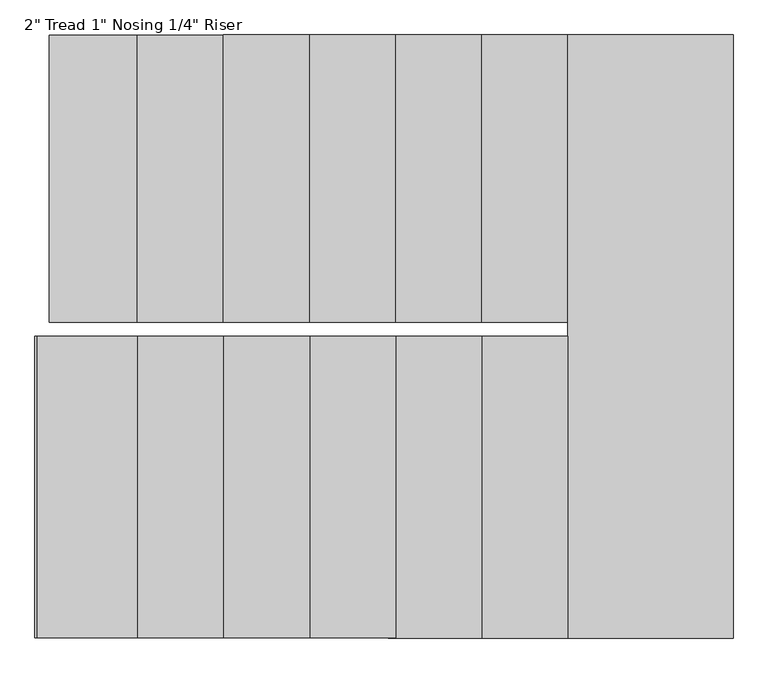
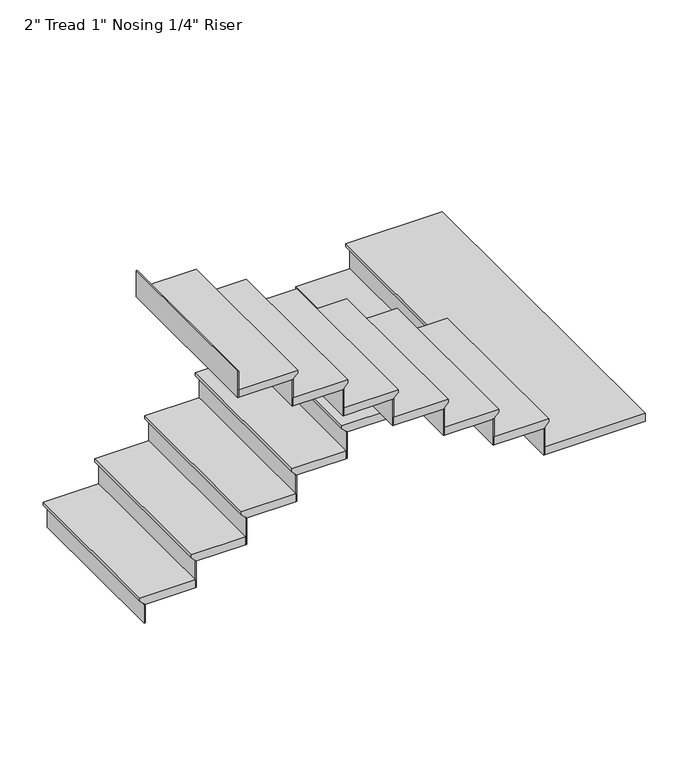
"""IFC4 building model written with IfcOpenShell, lengths in millimetres: stair flight geometry."""

from ifc_helpers import new_model, si_unit, origin, place, context, project, spatial, faceted_brep, source, transform, mapped, element, save


def stair_flight_5b4b54c9(model_context):
    return source(origin(), model_context, "Body", "Brep", [
        faceted_brep([(-1167.6638307, -167.7482799, 150.2833333), (-1167.6638307, -167.7482799, 169.3333333), (-1167.6638307, 848.2517201, 169.3333333), (-1167.6638307, 848.2517201, 150.2833333), (-1142.2638307, -167.7482799, 124.8833333), (-1142.2638307, 848.2517201, 124.8833333), (-831.1138307, -167.7482799, 169.3333333), (-831.1138307, 848.2517201, 169.3333333), (-1142.2638307, 848.2517201, 118.5333333), (-831.1138307, 848.2517201, 118.5333333), (-831.1138307, -167.7482799, 118.5333333), (-1142.2638307, -167.7482799, 118.5333333)], [[[0, 1, 2, 3]], [[4, 0, 3, 5]], [[2, 1, 6, 7]], [[8, 9, 10, 11]], [[2, 7, 9, 8, 5, 3]], [[8, 11, 4, 5]], [[6, 1, 0, 4, 11, 10]], [[7, 6, 10, 9]]]),
        faceted_brep([(-1142.2638307, -167.7482799, 118.5333333), (-1142.2638307, -167.7482799, 0.0), (-1135.9138307, -167.7482799, 0.0), (-1135.9138307, -167.7482799, 118.5333333), (-1142.2638307, 848.2517201, 118.5333333), (-1135.9138307, 848.2517201, 118.5333333), (-1135.9138307, 848.2517201, 0.0), (-1142.2638307, 848.2517201, 0.0)], [[[0, 1, 2, 3]], [[4, 5, 6, 7]], [[1, 0, 4, 7]], [[2, 1, 7, 6]], [[3, 2, 6, 5]], [[0, 3, 5, 4]]]),
        faceted_brep([(-831.1138307, -167.7482799, 287.8666667), (-831.1138307, -167.7482799, 118.5333333), (-824.7638307, -167.7482799, 118.5333333), (-824.7638307, -167.7482799, 287.8666667), (-831.1138307, 848.2517201, 287.8666667), (-824.7638307, 848.2517201, 287.8666667), (-824.7638307, 848.2517201, 118.5333333), (-831.1138307, 848.2517201, 118.5333333)], [[[0, 1, 2, 3]], [[4, 5, 6, 7]], [[1, 0, 4, 7]], [[2, 1, 7, 6]], [[3, 2, 6, 5]], [[0, 3, 5, 4]]]),
        faceted_brep([(-856.5138307, 848.2517201, 338.6666667), (-856.5138307, -167.7482799, 338.6666667), (-526.3138307, -167.7482799, 338.6666667), (-526.3138307, 848.2517201, 338.6666667), (-831.1138307, 848.2517201, 287.8666667), (-526.3138307, 848.2517201, 287.8666667), (-526.3138307, -167.7482799, 287.8666667), (-831.1138307, -167.7482799, 287.8666667), (-831.1138307, 848.2517201, 294.2166667), (-856.5138307, 848.2517201, 319.6166667), (-831.1138307, -167.7482799, 294.2166667), (-856.5138307, -167.7482799, 319.6166667)], [[[0, 1, 2, 3]], [[4, 5, 6, 7]], [[0, 3, 5, 4, 8, 9]], [[4, 7, 10, 8]], [[2, 1, 11, 10, 7, 6]], [[3, 2, 6, 5]], [[11, 1, 0, 9]], [[10, 11, 9, 8]]]),
        faceted_brep([(-526.3138307, -167.7482799, 457.2), (-526.3138307, -167.7482799, 287.8666667), (-519.9638307, -167.7482799, 287.8666667), (-519.9638307, -167.7482799, 457.2), (-526.3138307, 848.2517201, 457.2), (-519.9638307, 848.2517201, 457.2), (-519.9638307, 848.2517201, 287.8666667), (-526.3138307, 848.2517201, 287.8666667)], [[[0, 1, 2, 3]], [[4, 5, 6, 7]], [[1, 0, 4, 7]], [[2, 1, 7, 6]], [[3, 2, 6, 5]], [[0, 3, 5, 4]]]),
        faceted_brep([(-551.7138307, 848.2517201, 508.0), (-551.7138307, -167.7482799, 508.0), (-221.5138307, -167.7482799, 508.0), (-221.5138307, 848.2517201, 508.0), (-526.3138307, 848.2517201, 457.2), (-221.5138307, 848.2517201, 457.2), (-221.5138307, -167.7482799, 457.2), (-526.3138307, -167.7482799, 457.2), (-526.3138307, 848.2517201, 463.55), (-551.7138307, 848.2517201, 488.95), (-526.3138307, -167.7482799, 463.55), (-551.7138307, -167.7482799, 488.95)], [[[0, 1, 2, 3]], [[4, 5, 6, 7]], [[0, 3, 5, 4, 8, 9]], [[4, 7, 10, 8]], [[2, 1, 11, 10, 7, 6]], [[3, 2, 6, 5]], [[11, 1, 0, 9]], [[10, 11, 9, 8]]]),
        faceted_brep([(-221.5138307, -167.7482799, 626.5333333), (-221.5138307, -167.7482799, 457.2), (-215.1638307, -167.7482799, 457.2), (-215.1638307, -167.7482799, 626.5333333), (-221.5138307, 848.2517201, 626.5333333), (-215.1638307, 848.2517201, 626.5333333), (-215.1638307, 848.2517201, 457.2), (-221.5138307, 848.2517201, 457.2)], [[[0, 1, 2, 3]], [[4, 5, 6, 7]], [[1, 0, 4, 7]], [[2, 1, 7, 6]], [[3, 2, 6, 5]], [[0, 3, 5, 4]]]),
        faceted_brep([(-246.9138307, 848.2517201, 677.3333333), (-246.9138307, -167.7482799, 677.3333333), (83.2861693, -167.7482799, 677.3333333), (83.2861693, 848.2517201, 677.3333333), (-221.5138307, 848.2517201, 626.5333333), (83.2861693, 848.2517201, 626.5333333), (83.2861693, -167.7482799, 626.5333333), (-221.5138307, -167.7482799, 626.5333333), (-221.5138307, 848.2517201, 632.8833333), (-246.9138307, 848.2517201, 658.2833333), (-221.5138307, -167.7482799, 632.8833333), (-246.9138307, -167.7482799, 658.2833333)], [[[0, 1, 2, 3]], [[4, 5, 6, 7]], [[0, 3, 5, 4, 8, 9]], [[4, 7, 10, 8]], [[2, 1, 11, 10, 7, 6]], [[3, 2, 6, 5]], [[11, 1, 0, 9]], [[10, 11, 9, 8]]]),
        faceted_brep([(83.2861693, -167.7482799, 795.8666667), (83.2861693, -167.7482799, 626.5333333), (89.6361693, -167.7482799, 626.5333333), (89.6361693, -167.7482799, 795.8666667), (83.2861693, 848.2517201, 795.8666667), (89.6361693, 848.2517201, 795.8666667), (89.6361693, 848.2517201, 626.5333333), (83.2861693, 848.2517201, 626.5333333)], [[[0, 1, 2, 3]], [[4, 5, 6, 7]], [[1, 0, 4, 7]], [[2, 1, 7, 6]], [[3, 2, 6, 5]], [[0, 3, 5, 4]]]),
        faceted_brep([(57.8861693, 848.2517201, 846.6666667), (57.8861693, -167.7482799, 846.6666667), (388.0861693, -167.7482799, 846.6666667), (388.0861693, 848.2517201, 846.6666667), (83.2861693, 848.2517201, 795.8666667), (388.0861693, 848.2517201, 795.8666667), (388.0861693, -167.7482799, 795.8666667), (83.2861693, -167.7482799, 795.8666667), (83.2861693, 848.2517201, 802.2166667), (57.8861693, 848.2517201, 827.6166667), (83.2861693, -167.7482799, 802.2166667), (57.8861693, -167.7482799, 827.6166667)], [[[0, 1, 2, 3]], [[4, 5, 6, 7]], [[0, 3, 5, 4, 8, 9]], [[4, 7, 10, 8]], [[2, 1, 11, 10, 7, 6]], [[3, 2, 6, 5]], [[11, 1, 0, 9]], [[10, 11, 9, 8]]]),
        faceted_brep([(388.0861693, -167.7482799, 965.2), (388.0861693, -167.7482799, 795.8666667), (394.4361693, -167.7482799, 795.8666667), (394.4361693, -167.7482799, 965.2), (388.0861693, 848.2517201, 965.2), (394.4361693, 848.2517201, 965.2), (394.4361693, 848.2517201, 795.8666667), (388.0861693, 848.2517201, 795.8666667)], [[[0, 1, 2, 3]], [[4, 5, 6, 7]], [[1, 0, 4, 7]], [[2, 1, 7, 6]], [[3, 2, 6, 5]], [[0, 3, 5, 4]]]),
        faceted_brep([(362.6861693, 848.2517201, 1016.0), (362.6861693, -167.7482799, 1016.0), (692.8861693, -167.7482799, 1016.0), (692.8861693, 848.2517201, 1016.0), (388.0861693, 848.2517201, 965.2), (692.8861693, 848.2517201, 965.2), (692.8861693, -167.7482799, 965.2), (388.0861693, -167.7482799, 965.2), (388.0861693, 848.2517201, 971.55), (362.6861693, 848.2517201, 996.95), (388.0861693, -167.7482799, 971.55), (362.6861693, -167.7482799, 996.95)], [[[0, 1, 2, 3]], [[4, 5, 6, 7]], [[0, 3, 5, 4, 8, 9]], [[4, 7, 10, 8]], [[2, 1, 11, 10, 7, 6]], [[3, 2, 6, 5]], [[11, 1, 0, 9]], [[10, 11, 9, 8]]]),
        faceted_brep([(692.8861693, -167.7482799, 1134.5333333), (692.8861693, -167.7482799, 965.2), (699.2361693, -167.7482799, 965.2), (699.2361693, -167.7482799, 1134.5333333), (692.8861693, 848.2517201, 1134.5333333), (699.2361693, 848.2517201, 1134.5333333), (699.2361693, 848.2517201, 965.2), (692.8861693, 848.2517201, 965.2)], [[[0, 1, 2, 3]], [[4, 5, 6, 7]], [[1, 0, 4, 7]], [[2, 1, 7, 6]], [[3, 2, 6, 5]], [[0, 3, 5, 4]]]),
        faceted_brep([(642.0861693, -1285.3482799, 1185.3333333), (1251.6861693, -1285.3482799, 1185.3333333), (1251.6861693, 848.2517201, 1185.3333333), (667.4861693, 848.2517201, 1185.3333333), (667.4861693, -218.5482799, 1185.3333333), (642.0861693, -218.5482799, 1185.3333333), (1251.6861693, -1285.3482799, 1134.5333333), (642.0861693, -1285.3482799, 1134.5333333), (642.0861693, -218.5482799, 1134.5333333), (667.4861693, -218.5482799, 1134.5333333), (667.4861693, -167.7482799, 1134.5333333), (692.8861693, -167.7482799, 1134.5333333), (692.8861693, 848.2517201, 1134.5333333), (1251.6861693, 848.2517201, 1134.5333333), (692.8861693, 848.2517201, 1140.8833333), (667.4861693, 848.2517201, 1166.2833333), (692.8861693, -167.7482799, 1140.8833333), (667.4861693, -167.7482799, 1166.2833333)], [[[0, 1, 2, 3, 4, 5]], [[6, 7, 8, 9, 10, 11, 12, 13]], [[1, 0, 7, 6]], [[2, 1, 6, 13]], [[3, 2, 13, 12, 14, 15]], [[12, 11, 16, 14]], [[11, 10, 17, 16]], [[4, 3, 15, 17, 10, 9]], [[5, 4, 9, 8]], [[0, 5, 8, 7]], [[15, 14, 16, 17]]]),
        faceted_brep([(642.0861693, -218.5482799, 1303.8666667), (642.0861693, -218.5482799, 1134.5333333), (635.7361693, -218.5482799, 1134.5333333), (635.7361693, -218.5482799, 1303.8666667), (642.0861693, -1285.3482799, 1303.8666667), (635.7361693, -1285.3482799, 1303.8666667), (635.7361693, -1285.3482799, 1134.5333333), (642.0861693, -1285.3482799, 1134.5333333)], [[[0, 1, 2, 3]], [[4, 5, 6, 7]], [[1, 0, 4, 7]], [[2, 1, 7, 6]], [[3, 2, 6, 5]], [[0, 3, 5, 4]]]),
        faceted_brep([(667.4861693, -1285.3482799, 1354.6666667), (667.4861693, -218.5482799, 1354.6666667), (337.2861693, -218.5482799, 1354.6666667), (337.2861693, -1285.3482799, 1354.6666667), (642.0861693, -1285.3482799, 1303.8666667), (337.2861693, -1285.3482799, 1303.8666667), (337.2861693, -218.5482799, 1303.8666667), (642.0861693, -218.5482799, 1303.8666667), (642.0861693, -1285.3482799, 1310.2166667), (667.4861693, -1285.3482799, 1335.6166667), (642.0861693, -218.5482799, 1310.2166667), (667.4861693, -218.5482799, 1335.6166667)], [[[0, 1, 2, 3]], [[4, 5, 6, 7]], [[0, 3, 5, 4, 8, 9]], [[4, 7, 10, 8]], [[2, 1, 11, 10, 7, 6]], [[3, 2, 6, 5]], [[11, 1, 0, 9]], [[10, 11, 9, 8]]]),
        faceted_brep([(337.2861693, -218.5482799, 1473.2), (337.2861693, -218.5482799, 1303.8666667), (330.9361693, -218.5482799, 1303.8666667), (330.9361693, -218.5482799, 1473.2), (337.2861693, -1285.3482799, 1473.2), (330.9361693, -1285.3482799, 1473.2), (330.9361693, -1285.3482799, 1303.8666667), (337.2861693, -1285.3482799, 1303.8666667)], [[[0, 1, 2, 3]], [[4, 5, 6, 7]], [[1, 0, 4, 7]], [[2, 1, 7, 6]], [[3, 2, 6, 5]], [[0, 3, 5, 4]]]),
        faceted_brep([(362.6861693, -1285.3482799, 1524.0), (362.6861693, -218.5482799, 1524.0), (32.4861693, -218.5482799, 1524.0), (32.4861693, -1285.3482799, 1524.0), (337.2861693, -1285.3482799, 1473.2), (32.4861693, -1285.3482799, 1473.2), (32.4861693, -218.5482799, 1473.2), (337.2861693, -218.5482799, 1473.2), (337.2861693, -1285.3482799, 1479.55), (362.6861693, -1285.3482799, 1504.95), (337.2861693, -218.5482799, 1479.55), (362.6861693, -218.5482799, 1504.95)], [[[0, 1, 2, 3]], [[4, 5, 6, 7]], [[0, 3, 5, 4, 8, 9]], [[4, 7, 10, 8]], [[2, 1, 11, 10, 7, 6]], [[3, 2, 6, 5]], [[11, 1, 0, 9]], [[10, 11, 9, 8]]]),
        faceted_brep([(32.4861693, -218.5482799, 1642.5333333), (32.4861693, -218.5482799, 1473.2), (26.1361693, -218.5482799, 1473.2), (26.1361693, -218.5482799, 1642.5333333), (32.4861693, -1285.3482799, 1642.5333333), (26.1361693, -1285.3482799, 1642.5333333), (26.1361693, -1285.3482799, 1473.2), (32.4861693, -1285.3482799, 1473.2)], [[[0, 1, 2, 3]], [[4, 5, 6, 7]], [[1, 0, 4, 7]], [[2, 1, 7, 6]], [[3, 2, 6, 5]], [[0, 3, 5, 4]]]),
        faceted_brep([(57.8861693, -1285.3482799, 1693.3333333), (57.8861693, -218.5482799, 1693.3333333), (-272.3138307, -218.5482799, 1693.3333333), (-272.3138307, -1285.3482799, 1693.3333333), (32.4861693, -1285.3482799, 1642.5333333), (-272.3138307, -1285.3482799, 1642.5333333), (-272.3138307, -218.5482799, 1642.5333333), (32.4861693, -218.5482799, 1642.5333333), (32.4861693, -1285.3482799, 1648.8833333), (57.8861693, -1285.3482799, 1674.2833333), (32.4861693, -218.5482799, 1648.8833333), (57.8861693, -218.5482799, 1674.2833333)], [[[0, 1, 2, 3]], [[4, 5, 6, 7]], [[0, 3, 5, 4, 8, 9]], [[4, 7, 10, 8]], [[2, 1, 11, 10, 7, 6]], [[3, 2, 6, 5]], [[11, 1, 0, 9]], [[10, 11, 9, 8]]]),
        faceted_brep([(-272.3138307, -218.5482799, 1811.8666667), (-272.3138307, -218.5482799, 1642.5333333), (-278.6638307, -218.5482799, 1642.5333333), (-278.6638307, -218.5482799, 1811.8666667), (-272.3138307, -1285.3482799, 1811.8666667), (-278.6638307, -1285.3482799, 1811.8666667), (-278.6638307, -1285.3482799, 1642.5333333), (-272.3138307, -1285.3482799, 1642.5333333)], [[[0, 1, 2, 3]], [[4, 5, 6, 7]], [[1, 0, 4, 7]], [[2, 1, 7, 6]], [[3, 2, 6, 5]], [[0, 3, 5, 4]]]),
        faceted_brep([(-246.9138307, -1285.3482799, 1862.6666667), (-246.9138307, -218.5482799, 1862.6666667), (-577.1138307, -218.5482799, 1862.6666667), (-577.1138307, -1285.3482799, 1862.6666667), (-272.3138307, -1285.3482799, 1811.8666667), (-577.1138307, -1285.3482799, 1811.8666667), (-577.1138307, -218.5482799, 1811.8666667), (-272.3138307, -218.5482799, 1811.8666667), (-272.3138307, -1285.3482799, 1818.2166667), (-246.9138307, -1285.3482799, 1843.6166667), (-272.3138307, -218.5482799, 1818.2166667), (-246.9138307, -218.5482799, 1843.6166667)], [[[0, 1, 2, 3]], [[4, 5, 6, 7]], [[0, 3, 5, 4, 8, 9]], [[4, 7, 10, 8]], [[2, 1, 11, 10, 7, 6]], [[3, 2, 6, 5]], [[11, 1, 0, 9]], [[10, 11, 9, 8]]]),
        faceted_brep([(-577.1138307, -218.5482799, 1981.2), (-577.1138307, -218.5482799, 1811.8666667), (-583.4638307, -218.5482799, 1811.8666667), (-583.4638307, -218.5482799, 1981.2), (-577.1138307, -1285.3482799, 1981.2), (-583.4638307, -1285.3482799, 1981.2), (-583.4638307, -1285.3482799, 1811.8666667), (-577.1138307, -1285.3482799, 1811.8666667)], [[[0, 1, 2, 3]], [[4, 5, 6, 7]], [[1, 0, 4, 7]], [[2, 1, 7, 6]], [[3, 2, 6, 5]], [[0, 3, 5, 4]]]),
        faceted_brep([(-551.7138307, -1285.3482799, 2032.0), (-551.7138307, -218.5482799, 2032.0), (-881.9138307, -218.5482799, 2032.0), (-881.9138307, -1285.3482799, 2032.0), (-577.1138307, -1285.3482799, 1981.2), (-881.9138307, -1285.3482799, 1981.2), (-881.9138307, -218.5482799, 1981.2), (-577.1138307, -218.5482799, 1981.2), (-577.1138307, -1285.3482799, 1987.55), (-551.7138307, -1285.3482799, 2012.95), (-577.1138307, -218.5482799, 1987.55), (-551.7138307, -218.5482799, 2012.95)], [[[0, 1, 2, 3]], [[4, 5, 6, 7]], [[0, 3, 5, 4, 8, 9]], [[4, 7, 10, 8]], [[2, 1, 11, 10, 7, 6]], [[3, 2, 6, 5]], [[11, 1, 0, 9]], [[10, 11, 9, 8]]]),
        faceted_brep([(-881.9138307, -218.5482799, 2150.5333333), (-881.9138307, -218.5482799, 1981.2), (-888.2638307, -218.5482799, 1981.2), (-888.2638307, -218.5482799, 2150.5333333), (-881.9138307, -1285.3482799, 2150.5333333), (-888.2638307, -1285.3482799, 2150.5333333), (-888.2638307, -1285.3482799, 1981.2), (-881.9138307, -1285.3482799, 1981.2)], [[[0, 1, 2, 3]], [[4, 5, 6, 7]], [[1, 0, 4, 7]], [[2, 1, 7, 6]], [[3, 2, 6, 5]], [[0, 3, 5, 4]]]),
        faceted_brep([(-1212.1138307, -218.5482799, 2319.8666667), (-1212.1138307, -218.5482799, 2150.5333333), (-1218.4638307, -218.5482799, 2150.5333333), (-1218.4638307, -218.5482799, 2319.8666667), (-1212.1138307, -1285.3482799, 2319.8666667), (-1218.4638307, -1285.3482799, 2319.8666667), (-1218.4638307, -1285.3482799, 2150.5333333), (-1212.1138307, -1285.3482799, 2150.5333333)], [[[0, 1, 2, 3]], [[4, 5, 6, 7]], [[1, 0, 4, 7]], [[2, 1, 7, 6]], [[3, 2, 6, 5]], [[0, 3, 5, 4]]]),
        faceted_brep([(-856.5138307, -1285.3482799, 2201.3333333), (-856.5138307, -218.5482799, 2201.3333333), (-1212.1138307, -218.5482799, 2201.3333333), (-1212.1138307, -1285.3482799, 2201.3333333), (-881.9138307, -1285.3482799, 2150.5333333), (-1212.1138307, -1285.3482799, 2150.5333333), (-1212.1138307, -218.5482799, 2150.5333333), (-881.9138307, -218.5482799, 2150.5333333), (-881.9138307, -1285.3482799, 2156.8833333), (-856.5138307, -1285.3482799, 2182.2833333), (-881.9138307, -218.5482799, 2156.8833333), (-856.5138307, -218.5482799, 2182.2833333)], [[[0, 1, 2, 3]], [[4, 5, 6, 7]], [[0, 3, 5, 4, 8, 9]], [[4, 7, 10, 8]], [[2, 1, 11, 10, 7, 6]], [[3, 2, 6, 5]], [[11, 1, 0, 9]], [[10, 11, 9, 8]]]),
    ])


if __name__ == "__main__":
    model = new_model("IFC4")
    model_context = context("Model", 3, world=origin())
    ifc_project = project(units=[si_unit("LENGTHUNIT", "METRE", prefix="MILLI")], contexts=[model_context])
    site = spatial("IfcSite", under=ifc_project)
    building = spatial("IfcBuilding", under=site)
    placement = place(None, origin())
    stair_flight_shape = stair_flight_5b4b54c9(model_context)
    element("IfcStairFlight", 1, ObjectType="2\" Tread 1\" Nosing 1/4\" Riser", at=placement, inside=building, context=model_context, shape_type="MappedRepresentation", body=[
        mapped(stair_flight_shape, transform((0.0, 0.0, 0.0), x_axis=(1.0, 0.0, 0.0), y_axis=(0.0, 1.0, 0.0), z_axis=(0.0, 0.0, 1.0))),
    ])
    save(model, "model.ifc")
